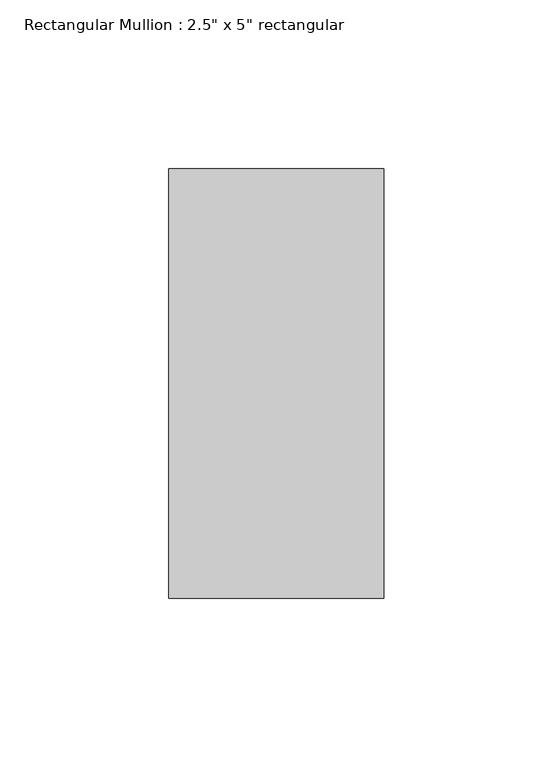
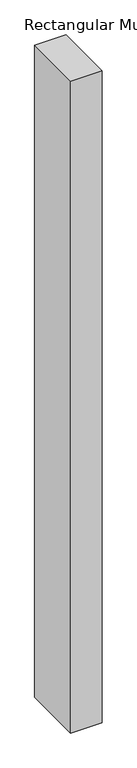
"""IFC4 building model written with IfcOpenShell, lengths in millimetres: member geometry."""

from ifc_helpers import new_model, si_unit, frame, origin, place, context, project, spatial, polyline, outline, extrude, source, transform, mapped, element, save


def member_41dcc1f0(model_context):
    return source(origin(), model_context, "Body", "SweptSolid", [
        extrude(outline(polyline([(31.75, 63.5), (31.75, -63.5), (-31.75, -63.5), (-31.75, 63.5), (31.75, 63.5)])), frame((0.0, 0.0, -1403.35), z_axis=(0.0, 0.0, 1.0), x_axis=(1.0, 0.0, 0.0)), (0.0, 0.0, 1.0), 1403.35),
    ])


if __name__ == "__main__":
    model = new_model("IFC4")
    model_context = context("Model", 3, world=origin())
    ifc_project = project(units=[si_unit("LENGTHUNIT", "METRE", prefix="MILLI")], contexts=[model_context])
    site = spatial("IfcSite", under=ifc_project)
    building = spatial("IfcBuilding", under=site)
    placement = place(None, origin())
    member_shape = member_41dcc1f0(model_context)
    element("IfcMember", 1, ObjectType="Rectangular Mullion : 2.5\" x 5\" rectangular", at=placement, inside=building, context=model_context, shape_type="MappedRepresentation", body=[
        mapped(member_shape, transform((0.0, 0.0, 0.0), x_axis=(1.0, 0.0, 0.0), y_axis=(0.0, 1.0, 0.0), z_axis=(0.0, 0.0, 1.0))),
    ])
    save(model, "model.ifc")

# Revit data of these elements
# Type "Rectangular Mullion : 2.5\" x 5\" rectangular"
#   built-in parameter 1007304 = 0.416667 (stored number, unit not read)
#   built-in parameter 1007301 = 0.104167 (stored number, unit not read)
#   built-in parameter 1007300 = 0.104167 (stored number, unit not read)
# Element 1 (IfcMember, "Rectangular Mullion : 2.5\" x 5\" rectangular")
#   Materials on its faces: "Aluminum"
# Materials
#   "Aluminum": class "Metal", colour RGB 247 247 247, transparency 0, Description = "Aluminum 6061", Cost = 0
